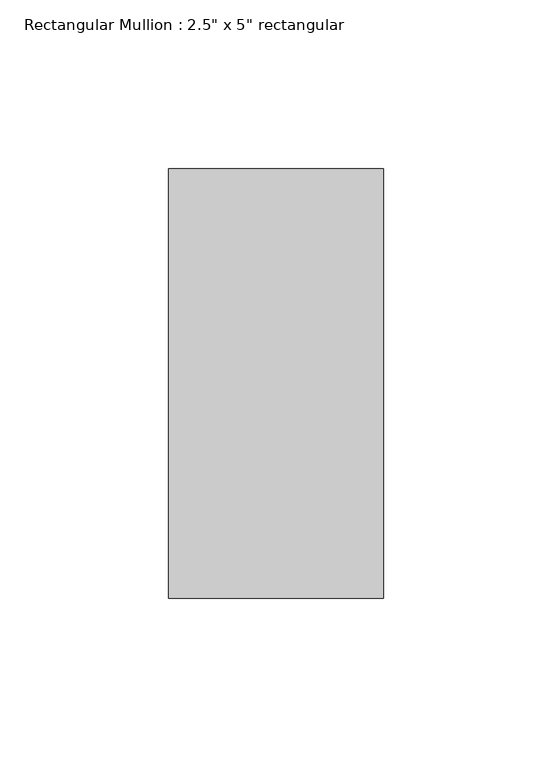
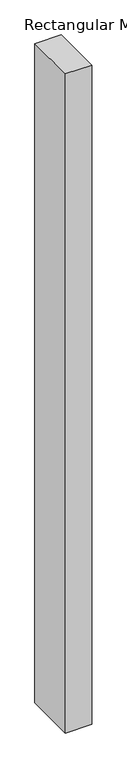
"""IFC4 building model written with IfcOpenShell, lengths in millimetres: member geometry."""

from ifc_helpers import new_model, si_unit, frame, origin, place, context, project, spatial, polyline, outline, extrude, source, transform, mapped, element, save


def member_38e9bff8(model_context):
    return source(origin(), model_context, "Body", "SweptSolid", [
        extrude(outline(polyline([(31.75, 63.5), (31.75, -63.5), (-31.75, -63.5), (-31.75, 63.5), (31.75, 63.5)])), frame((0.0, 0.0, -1676.4), z_axis=(0.0, 0.0, 1.0), x_axis=(1.0, 0.0, 0.0)), (0.0, 0.0, 1.0), 1676.4),
    ])


if __name__ == "__main__":
    model = new_model("IFC4")
    model_context = context("Model", 3, world=origin())
    ifc_project = project(units=[si_unit("LENGTHUNIT", "METRE", prefix="MILLI")], contexts=[model_context])
    site = spatial("IfcSite", under=ifc_project)
    building = spatial("IfcBuilding", under=site)
    placement = place(None, origin())
    member_shape = member_38e9bff8(model_context)
    element("IfcMember", 1, ObjectType="Rectangular Mullion : 2.5\" x 5\" rectangular", at=placement, inside=building, context=model_context, shape_type="MappedRepresentation", body=[
        mapped(member_shape, transform((0.0, 0.0, 0.0), x_axis=(1.0, 0.0, 0.0), y_axis=(0.0, 1.0, 0.0), z_axis=(0.0, 0.0, 1.0))),
    ])
    save(model, "model.ifc")

# Revit data of these elements
# Type "Rectangular Mullion : 2.5\" x 5\" rectangular"
#   built-in parameter 1007304 = 0.416667 (stored number, unit not read)
#   built-in parameter 1007301 = 0.104167 (stored number, unit not read)
#   built-in parameter 1007300 = 0.104167 (stored number, unit not read)
